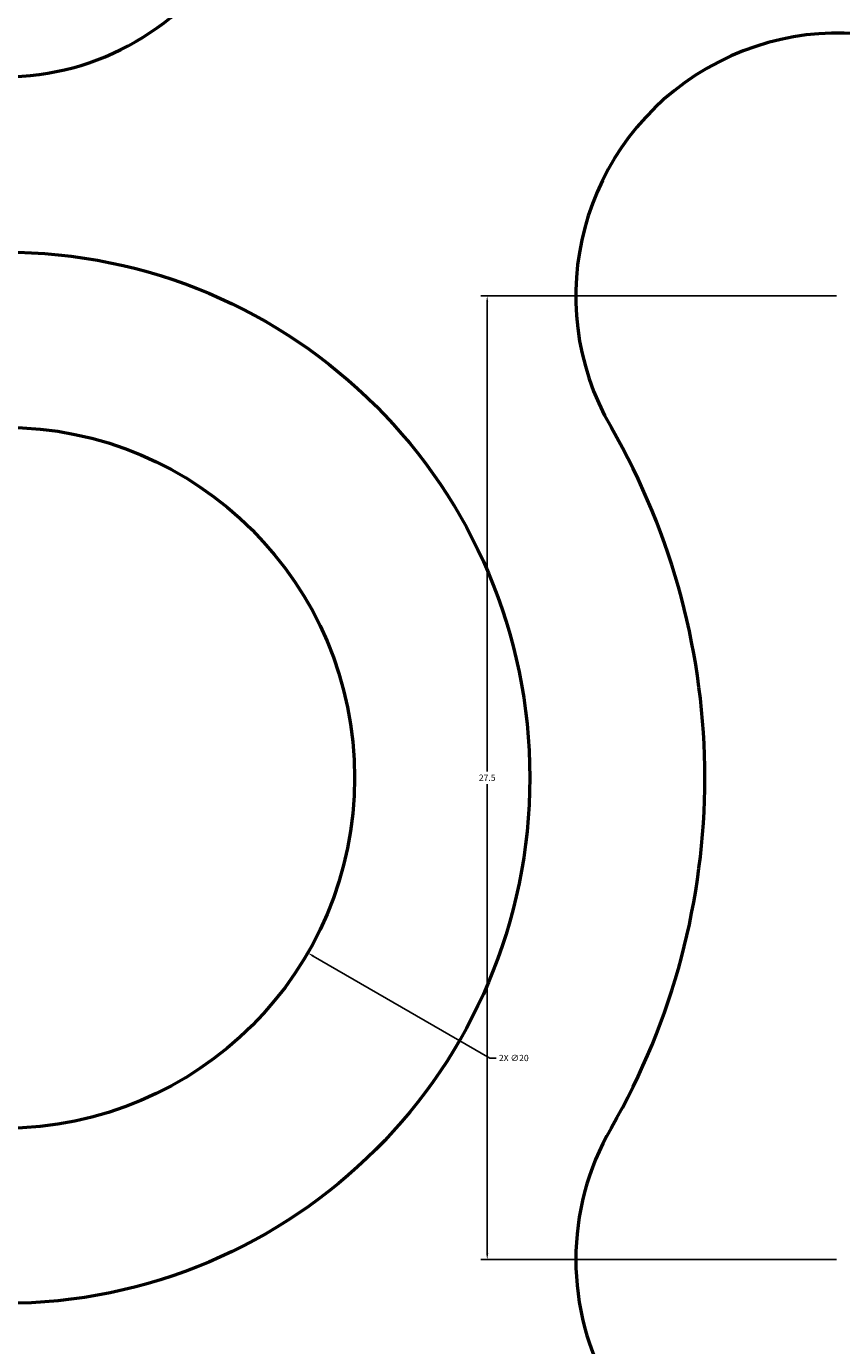
# Model space of a CAD drawing. Units: inches. Extents: x 413 to 622, y 326 to 447.
# Tile 5 of 15: x 473 to 497, y 370 to 408. Entities that reach past the tile are written whole.
import ezdxf

# ---------------------------------------------------------------- set-up
doc = ezdxf.new("R2010")
doc.units = ezdxf.units.IN
doc.header["$MEASUREMENT"] = 0
doc.layers.add('M-DIMS', color=2, linetype='Continuous', lineweight=18)
doc.layers.add('M-OUTL', color=7, linetype='Continuous', lineweight=50)
doc.styles.get("Standard").update_dxf_attribs({"font": 'arial.ttf'})
doc.dimstyles.get("Standard").update_dxf_attribs({"dimtxt": 0.18, "dimasz": 0.18, "dimexe": 0.18, "dimexo": 0.0625, "dimgap": 0.09, "dimtad": 0, "dimtih": 1, "dimtoh": 1, "dimdec": 4, "dimzin": 0, "dimdsep": 46, "dimtxsty": 'Standard', "dimcen": 0.09, "dimadec": 0, "dimazin": 0, "dimtfac": 1, "dimtdec": 4, "dimtofl": 0, "dimtmove": 0, "dimatfit": 3, "dimfxl": 1, "dimtolj": 1, "dimtzin": 0, "dimarcsym": 0})

# ---------------------------------------------------------------- blocks, each defined once
blk = doc.blocks.new('SPROCKET-HUB-BORE')
for radius in [15, 10]:
    blk.add_circle((15, 15), radius)
blk = doc.blocks.new('SPROCKET-WEB-SLOT')
for centre, radius, start, end in [((7.501, 21.25), 7.5, 30, 210), ((31.317, 35), 20, 210, 270), ((31.317, 35), 35, 210, 270), ((31.317, 7.5), 7.5, 270, 90)]:
    blk.add_arc(centre, radius, start, end)
blk = doc.blocks.new('*D11')
at = {"layer": 'Defpoints', "color": 0, "transparency": 16777216}
for p in [(621.66, 446.422), (621.66, 388.074), (423.314, 378.888)]:
    blk.add_point(p, dxfattribs=at)
at = {"layer": 'M-DIMS', "color": 0, "lineweight": -2, "transparency": 16777216}
for p, q in [((423.314, 378.95), (423.314, 446.602)), ((621.66, 388.137), (621.66, 446.602)), ((423.494, 446.422), (522.031, 446.422)), ((621.48, 446.422), (522.943, 446.422))]:
    blk.add_line(p, q, dxfattribs=at)
at = {"layer": 'M-DIMS', "color": 0, "transparency": 16777216}
for points in [[(423.494, 446.452), (423.494, 446.392), (423.314, 446.422)], [(621.48, 446.452), (621.48, 446.392), (621.66, 446.422)]]:
    blk.add_solid(points, dxfattribs=at)
at = {"layer": 'M-DIMS', "color": 0, "transparency": 16777216, "insert": (522.487, 446.422), "char_height": 0.18, "attachment_point": 5}
blk.add_mtext('\\A1;198.35', dxfattribs=at)
blk = doc.blocks.new('*D12')
at = {"layer": 'Defpoints', "color": 0, "transparency": 16777216}
for p in [(472.684, 386.392), (592.684, 386.392), (592.684, 326.361)]:
    blk.add_point(p, dxfattribs=at)
at = {"layer": 'M-DIMS', "color": 0, "lineweight": -2, "transparency": 16777216}
for p, q in [((472.684, 386.329), (472.684, 326.181)), ((592.684, 386.329), (592.684, 326.181)), ((472.864, 326.361), (532.404, 326.361)), ((592.504, 326.361), (532.964, 326.361))]:
    blk.add_line(p, q, dxfattribs=at)
at = {"layer": 'M-DIMS', "color": 0, "transparency": 16777216}
for points in [[(472.864, 326.391), (472.864, 326.331), (472.684, 326.361)], [(592.504, 326.391), (592.504, 326.331), (592.684, 326.361)]]:
    blk.add_solid(points, dxfattribs=at)
at = {"layer": 'M-DIMS', "color": 0, "transparency": 16777216, "insert": (532.684, 326.361), "char_height": 0.18, "attachment_point": 5}
blk.add_mtext('\\A1;120', dxfattribs=at)
blk = doc.blocks.new('*D14')
at = {"layer": 'Defpoints', "color": 0, "transparency": 16777216}
for p in [(486.469, 400.142), (496.499, 400.142), (496.499, 372.642)]:
    blk.add_point(p, dxfattribs=at)
at = {"layer": 'M-DIMS', "color": 0, "lineweight": -2, "transparency": 16777216}
for p, q in [((496.437, 400.142), (486.289, 400.142)), ((486.469, 399.962), (486.469, 386.573)), ((486.469, 372.822), (486.469, 386.21)), ((496.437, 372.642), (486.289, 372.642))]:
    blk.add_line(p, q, dxfattribs=at)
at = {"layer": 'M-DIMS', "color": 0, "transparency": 16777216}
for points in [[(486.439, 399.962), (486.499, 399.962), (486.469, 400.142)], [(486.439, 372.822), (486.499, 372.822), (486.469, 372.642)]]:
    blk.add_solid(points, dxfattribs=at)
at = {"layer": 'M-DIMS', "color": 0, "transparency": 16777216, "insert": (486.469, 386.392), "char_height": 0.18, "attachment_point": 5}
blk.add_mtext('\\A1;27.5', dxfattribs=at)
blk = doc.blocks.new('*D24')
at = {"layer": 'Defpoints', "color": 0, "transparency": 16777216}
for p in [(432.684, 386.391), (512.684, 386.392)]:
    blk.add_point(p, dxfattribs=at)
at = {"layer": 'M-DIMS', "color": 0, "lineweight": -2, "transparency": 16777216}
for p, q in [((472.594, 386.392), (472.774, 386.392)), ((472.684, 386.302), (472.684, 386.482)), ((536.684, 386.392), (512.864, 386.392))]:
    blk.add_line(p, q, dxfattribs=at)
at = {"layer": 'M-DIMS', "color": 0, "transparency": 16777216}
blk.add_solid([(512.864, 386.422), (512.864, 386.362), (512.684, 386.392)], dxfattribs=at)
at = {"layer": 'M-DIMS', "color": 0, "transparency": 16777216, "insert": (537, 386.392), "char_height": 0.18, "attachment_point": 5}
blk.add_mtext('\\A1;∅80', dxfattribs=at)
blk = doc.blocks.new('*D26')
at = {"layer": 'Defpoints', "color": 0, "transparency": 16777216}
for p in [(459.693, 393.89), (485.675, 378.893)]:
    blk.add_point(p, dxfattribs=at)
at = {"layer": 'M-DIMS', "color": 0, "lineweight": -2, "transparency": 16777216}
for p, q in [((451.718, 398.39), (451.898, 398.39)), ((451.898, 398.39), (459.537, 393.98)), ((472.594, 386.392), (472.774, 386.392)), ((472.684, 386.302), (472.684, 386.482))]:
    blk.add_line(p, q, dxfattribs=at)
at = {"layer": 'M-DIMS', "color": 0, "transparency": 16777216}
blk.add_solid([(459.552, 394.006), (459.522, 393.954), (459.693, 393.89)], dxfattribs=at)
at = {"layer": 'M-DIMS', "color": 0, "transparency": 16777216, "insert": (451.211, 398.39), "char_height": 0.18, "attachment_point": 5}
blk.add_mtext('\\A1;2X ∅30', dxfattribs=at)
blk = doc.blocks.new('*D27')
at = {"layer": 'Defpoints', "color": 0, "transparency": 16777216}
for p in [(464.022, 391.39), (481.345, 381.393)]:
    blk.add_point(p, dxfattribs=at)
at = {"layer": 'M-DIMS', "color": 0, "lineweight": -2, "transparency": 16777216}
for p, q in [((472.594, 386.392), (472.774, 386.392)), ((472.684, 386.302), (472.684, 386.482)), ((486.542, 378.394), (481.501, 381.303)), ((486.722, 378.394), (486.542, 378.394))]:
    blk.add_line(p, q, dxfattribs=at)
at = {"layer": 'M-DIMS', "color": 0, "transparency": 16777216}
blk.add_solid([(481.516, 381.329), (481.486, 381.277), (481.345, 381.393)], dxfattribs=at)
at = {"layer": 'M-DIMS', "color": 0, "transparency": 16777216, "insert": (487.228, 378.394), "char_height": 0.18, "attachment_point": 5}
blk.add_mtext('\\A1;2X ∅20', dxfattribs=at)

msp = doc.modelspace()

# ---------------------------------------------------------------- linework, layer by layer
at = {"layer": 'M-OUTL'}
msp.add_circle((472.6836, 386.3915), 40, dxfattribs=at)

# ---------------------------------------------------------------- block references
for p, rotation in [((458.0314, 431.0122), 239.9999999999996), ((518.6523, 376.7703), 119.9999999999996)]:
    msp.add_blockref('SPROCKET-WEB-SLOT', p, dxfattribs=dict(at, rotation=rotation))
for name, p in [('SPROCKET-HUB-BORE', (457.684, 371.392)), ('SPROCKET-WEB-SLOT', (441.367, 351.392))]:
    msp.add_blockref(name, p, dxfattribs=at)

# ---------------------------------------------------------------- dimensions: what is measured, and where the dimension line sits
at = {"layer": 'M-DIMS'}
for base, p1, p2, override, picture, middle in [((621.66, 446.422), (423.3136, 378.8878), (621.66, 388.0741), {"dimdec": 2, "dimlfac": 1, "dimrnd": 0, "dimzin": 0, "dimdsep": 46, "dimlunit": 2}, '*D11', (522.4868, 446.422)), ((592.6836, 326.361), (472.6836, 386.3915), (592.6836, 386.3915), {"dimdec": 0, "dimlfac": 1, "dimrnd": 0, "dimzin": 0, "dimdsep": 46, "dimlunit": 2}, '*D12', (532.6836, 326.361))]:
    dim = msp.add_linear_dim(base=base, p1=p1, p2=p2, dimstyle='Standard', override=override, dxfattribs=at)
    dim.commit()
    dim.dimension.update_dxf_attribs({"geometry": picture, "text_midpoint": middle})
dim = msp.add_linear_dim(base=(486.4688, 400.1415), p1=(496.4993, 372.6415), p2=(496.4993, 400.1415), angle=90, dimstyle='Standard', override={"dimdec": 1, "dimlfac": 1, "dimrnd": 0, "dimzin": 0, "dimdsep": 46, "dimlunit": 2}, dxfattribs=at)
dim.commit()
dim.dimension.update_dxf_attribs({"geometry": '*D14', "text_midpoint": (486.4688, 386.3915)})
for p1, p2, picture, middle in [((485.6746, 378.8925), (459.6926, 393.8905), '*D26', (451.2114, 398.3899)), ((464.0223, 391.3898), (481.3448, 381.3932), '*D27', (487.2283, 378.3943))]:
    dim = msp.add_diameter_dim_2p(p1=p1, p2=p2, text='2X <>', dimstyle='Standard', override={"dimdec": 0, "dimlfac": 1, "dimrnd": 0, "dimzin": 0, "dimdsep": 46, "dimlunit": 2}, dxfattribs=at)
    dim.commit()
    dim.dimension.update_dxf_attribs({"geometry": picture, "text_midpoint": middle, "dimtype": 163})
dim = msp.add_diameter_dim_2p(p1=(432.6836, 386.391), p2=(512.6836, 386.392), dimstyle='Standard', override={"dimdec": 0, "dimlfac": 1, "dimrnd": 0, "dimzin": 0, "dimdsep": 46, "dimlunit": 2}, dxfattribs=at)
dim.commit()
dim.dimension.update_dxf_attribs({"geometry": '*D24', "text_midpoint": (536.6836, 386.3923), "dimtype": 163})

doc.saveas('drawing.dxf')
